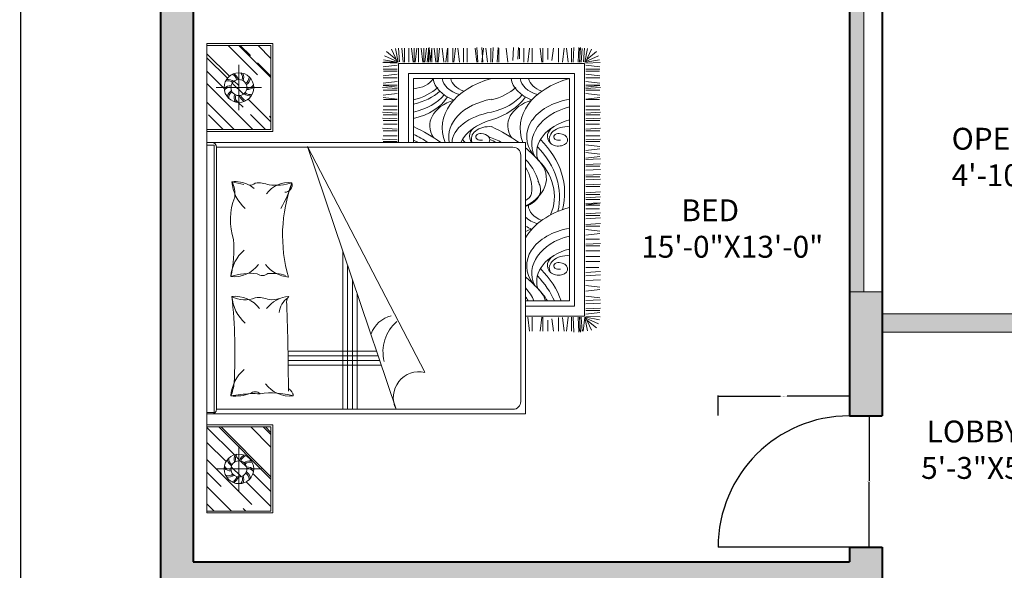
# Model space of a CAD drawing. Units: inches. Extents: x 2985 to 3527, y 3685 to 4528.
# Tile 3 of 5: x 2985 to 3255, y 4195 to 4346. Entities that reach past the tile are written whole.
import ezdxf

# ---------------------------------------------------------------- set-up
doc = ezdxf.new("R2010")
doc.units = ezdxf.units.IN
for name, color, linetype, lineweight in [('A-ANNO-DIMS', 2, 'Continuous', 18), ('A-AREA-IDEN', 7, 'Continuous', 25), ('A-FURN', 8, 'Continuous', 18), ('A-GLAZ', 4, 'Continuous', 18), ('A-WALL', 7, 'Continuous', 40), ('A-WALL-PATT', 8, 'Continuous', 13), ('door', 4, 'Continuous', 25)]:
    doc.layers.add(name, color=color, linetype=linetype, lineweight=lineweight)
doc.layers.add('A-GLAZ-PATT', color=241, linetype='Continuous', lineweight=13, true_color=0xf7abae)
doc.styles.get("Standard").update_dxf_attribs({"font": 'arial.ttf'})
doc.dimstyles.get("Standard").update_dxf_attribs({"dimtxt": 0.18, "dimasz": 0.18, "dimexe": 0.18, "dimexo": 0.0625, "dimgap": 0.09, "dimtad": 0, "dimtih": 1, "dimtoh": 1, "dimdec": 4, "dimzin": 0, "dimdsep": 46, "dimtxsty": 'Standard', "dimcen": 0.09, "dimadec": 0, "dimazin": 0, "dimtfac": 1, "dimtdec": 4, "dimtofl": 0, "dimtmove": 0, "dimatfit": 3, "dimfxl": 1, "dimtolj": 1, "dimtzin": 0, "dimarcsym": 0})

# ---------------------------------------------------------------- blocks, each defined once
blk = doc.blocks.new('A$C64B41DC1')
for p, q in [((0, 2.5079), (2.9903, 2.5079)), ((0, 2.0879), (0, 2.5079)), ((0.012, 2.4618), (0.0581, 2.5079)), ((0.012, 2.3515), (0.1684, 2.5079)), ((0.012, 2.0999), (0.012, 2.5079)), ((0.0543, 2.2213), (0.3409, 2.5079)), ((0.1689, 2.4179), (0.2589, 2.5079)), ((0.2804, 2.1597), (0.2804, 2.4481)), ((0.3265, 2.386), (0.4484, 2.5079)), ((0.3699, 2.3332), (0.5445, 2.5079)), ((0.548, 2.5079), (0.548, 2.0999)), ((0.56, 2.5079), (0.56, 2.0879)), ((0.6301, 2.5079), (0.6301, 0.4779)), ((0.6401, 2.461), (0.6401, 2.5079)), ((0.6401, 2.5079), (2.344, 2.5079)), ((2.344, 2.461), (0.6401, 2.461)), ((2.344, 2.5079), (2.3601, 2.5079)), ((2.344, 2.5079), (2.344, 2.461)), ((2.3601, 2.5079), (2.3601, 2.4761)), ((2.3601, 0.4779), (2.3601, 2.5079)), ((2.4303, 2.5079), (2.4303, 2.0879)), ((2.4423, 2.5079), (2.4423, 2.0999)), ((2.4423, 2.3333), (2.6169, 2.5079)), ((2.4423, 2.2145), (2.7357, 2.5079)), ((2.4423, 2.404), (2.5354, 2.4971)), ((2.705, 2.398), (2.8149, 2.5079)), ((2.7099, 2.1597), (2.7099, 2.4481)), ((2.7691, 2.3772), (2.8998, 2.5079)), ((2.7819, 2.3646), (2.9252, 2.5079)), ((2.9783, 2.0999), (2.9783, 2.5079)), ((2.9903, 2.0879), (2.9903, 2.5079)), ((0.2157, 2.0999), (0.548, 2.4322)), ((0.2299, 2.0999), (0.548, 2.418)), ((0.6601, 2.4461), (1.4951, 2.4461)), ((0.6601, 2.4461), (0.6601, 0.5579)), ((1.4951, 2.4461), (0.6697, 2.4461)), ((2.3301, 2.4461), (1.4951, 2.4461)), ((2.3301, 0.5579), (2.3301, 2.4461)), ((0.2311, 2.2906), (0.2937, 2.3532)), ((0.3405, 2.3039), (0.3605, 2.3238)), ((2.6158, 2.3088), (2.6313, 2.3243)), ((2.6674, 2.2756), (2.7382, 2.3464)), ((2.7249, 2.3076), (2.7512, 2.3339)), ((2.7914, 2.1846), (2.9783, 2.3715)), ((0.012, 2.261), (0.0275, 2.2765)), ((0.1362, 2.3039), (0.4246, 2.3039)), ((0.2905, 2.2539), (0.3304, 2.2938)), ((2.8541, 2.3039), (2.5657, 2.3039)), ((2.5849, 2.2779), (2.6158, 2.3088)), ((2.7746, 2.0999), (2.9783, 2.3036)), ((2.9144, 2.2312), (2.9783, 2.2951)), ((0.0404, 2.0999), (0.1982, 2.2578)), ((0.1365, 2.0999), (0.251, 2.2144)), ((0.4194, 2.0999), (0.548, 2.2285)), ((2.4423, 2.1353), (2.5382, 2.2312)), ((2.4918, 2.0999), (2.6366, 2.2447)), ((0.4986, 2.0999), (0.548, 2.1493)), ((0.5127, 2.0999), (0.548, 2.1352)), ((2.7831, 2.0999), (2.8678, 2.1846)), ((2.8962, 2.0999), (2.9783, 2.182)), ((0.56, 2.0879), (0, 2.0879)), ((0.548, 2.0999), (0.012, 2.0999)), ((2.4303, 2.0879), (2.9903, 2.0879)), ((2.4423, 2.0999), (2.9783, 2.0999)), ((2.5172, 2.0999), (2.5269, 2.1096)), ((0.9415, 1.9902), (0.9415, 1.3975)), ((0.9715, 1.9906), (0.9715, 1.4076)), ((1.0015, 1.991), (1.0015, 1.4177)), ((1.0315, 1.9916), (1.0315, 1.4279)), ((2.3349, 1.8678), (0.6613, 1.3029)), ((0.8956, 1.1191), (2.3349, 1.8678)), ((1.6636, 1.6412), (0.6601, 1.6412)), ((1.5748, 1.6112), (0.6601, 1.6112)), ((2.3665, 1.295), (2.3665, 1.3839)), ((2.377, 1.295), (2.3822, 1.3891)), ((2.4032, 1.295), (2.4032, 1.3839)), ((2.4346, 1.295), (2.4346, 1.3839)), ((2.4451, 1.295), (2.4503, 1.3891)), ((2.4774, 1.2957), (2.4774, 1.3837)), ((2.5, 1.295), (2.5, 1.3839)), ((2.5105, 1.295), (2.5157, 1.3891)), ((2.5367, 1.295), (2.5367, 1.3839)), ((2.5471, 1.295), (2.5524, 1.3891)), ((2.5681, 1.295), (2.5681, 1.3839)), ((2.5918, 1.295), (2.5918, 1.3839)), ((2.6346, 1.2957), (2.6346, 1.3837)), ((2.6362, 1.2957), (2.6467, 1.3839)), ((2.6729, 1.295), (2.6624, 1.3839)), ((2.6938, 1.295), (2.6938, 1.3839)), ((2.7043, 1.295), (2.7095, 1.3891)), ((2.7127, 1.2957), (2.7232, 1.3839)), ((2.7253, 1.295), (2.7253, 1.3839)), ((2.7494, 1.295), (2.7389, 1.3839)), ((2.7718, 1.295), (2.7718, 1.3839)), ((2.7959, 1.295), (2.7854, 1.3839)), ((2.8146, 1.2957), (2.8146, 1.3837)), ((2.8146, 1.2957), (2.8146, 1.3837)), ((2.8282, 1.295), (2.8282, 1.3839)), ((2.8282, 1.295), (2.8282, 1.3839)), ((2.8523, 1.295), (2.8418, 1.3839)), ((2.8523, 1.295), (2.8418, 1.3839)), ((2.8653, 1.2966), (2.8688, 1.3861)), ((2.8711, 1.2957), (2.8711, 1.3837)), ((2.8711, 1.2957), (2.8875, 1.3822)), ((2.8713, 1.2927), (2.954, 1.3315)), ((2.8765, 1.2958), (2.9132, 1.3758)), ((2.8893, 1.3011), (2.9394, 1.3636)), ((2.3601, 1.2873), (2.8639, 1.2873)), ((2.8639, 1.2873), (2.8639, 0.1018)), ((2.8716, 1.2565), (2.9605, 1.2669)), ((2.8717, 1.2884), (2.9588, 1.3058)), ((2.8744, 1.2817), (2.9603, 1.2869)), ((2.3601, 1.2233), (2.7999, 1.2233)), ((2.7999, 1.2233), (2.7999, 0.1658)), ((2.8716, 1.2212), (2.9605, 1.2212)), ((2.8716, 1.1947), (2.9605, 1.2052)), ((2.8723, 1.2489), (2.9603, 1.2489)), ((2.3601, 1.1913), (2.7679, 1.1912)), ((2.7679, 1.1912), (2.7679, 0.1978)), ((2.8716, 1.181), (2.9605, 1.1705)), ((2.8716, 1.1595), (2.9605, 1.1595)), ((2.8716, 1.133), (2.9605, 1.1435)), ((2.8723, 1.1872), (2.9603, 1.1872)), ((2.8716, 1.1193), (2.9605, 1.1088)), ((2.8716, 1.1035), (2.9605, 1.093)), ((2.8716, 1.0965), (2.9605, 1.0965)), ((2.8716, 1.086), (2.9657, 1.0913)), ((2.8716, 1.0756), (2.9605, 1.0756)), ((2.8723, 1.1255), (2.9603, 1.1255)), ((2.8723, 1.0858), (2.9605, 1.0753)), ((2.8716, 1.0491), (2.9605, 1.0596)), ((2.8716, 1.0354), (2.9605, 1.0249)), ((2.8723, 1.0416), (2.9603, 1.0416)), ((2.8723, 0.9987), (2.9605, 1.0092)), ((2.8723, 0.985), (2.9605, 0.9745)), ((2.8723, 0.9735), (2.9603, 0.9735)), ((2.8716, 0.9346), (2.9605, 0.9241)), ((2.8723, 0.9408), (2.9603, 0.9408)), ((2.8723, 0.8979), (2.9605, 0.9084)), ((2.8723, 0.8726), (2.9603, 0.8726)), ((2.8723, 0.8505), (2.9603, 0.8505)), ((2.8716, 0.7885), (2.9605, 0.799)), ((2.8716, 0.7818), (2.9657, 0.787)), ((2.8716, 0.7503), (2.9657, 0.7556)), ((2.8723, 0.7571), (2.9605, 0.7466)), ((2.8716, 0.7204), (2.9605, 0.7309)), ((2.8716, 0.6995), (2.9605, 0.6995)), ((2.8716, 0.689), (2.9657, 0.6838)), ((2.8716, 0.6576), (2.9657, 0.6523)), ((2.8716, 0.6471), (2.9605, 0.6471)), ((2.8716, 0.5903), (2.9605, 0.6007)), ((0.7101, 0.5079), (2.2801, 0.5079)), ((2.882, 0.5582), (2.9657, 0.5536)), ((2.8909, 0.5263), (2.9657, 0.5222)), ((2.8928, 0.5169), (2.9605, 0.5169)), ((0.6301, 0.4779), (2.3601, 0.4779)), ((1.2465, 0.4625), (1.1576, 0.452)), ((1.2542, 0.1018), (1.2542, 0.4779)), ((1.3182, 0.1658), (1.3182, 0.4779)), ((1.3502, 0.1978), (1.3502, 0.4779)), ((2.8716, 0.4877), (2.9603, 0.4877)), ((2.8716, 0.4625), (2.9605, 0.452)), ((1.2465, 0.3746), (1.1576, 0.3851)), ((1.2465, 0.4365), (1.1577, 0.4365)), ((2.8716, 0.4365), (2.9603, 0.4365)), ((2.8716, 0.3746), (2.9605, 0.3851)), ((1.2465, 0.3684), (1.1577, 0.3684)), ((1.2285, 0.3357), (1.1577, 0.3357)), ((2.8716, 0.3684), (2.9603, 0.3684)), ((2.8896, 0.3357), (2.9603, 0.3357)), ((1.2355, 0.3092), (1.1576, 0.3)), ((1.2457, 0.2676), (1.1577, 0.2676)), ((2.8723, 0.2676), (2.9603, 0.2676)), ((2.8826, 0.3092), (2.9605, 0.3)), ((1.2457, 0.2423), (1.1576, 0.2319)), ((1.2465, 0.2057), (1.1576, 0.2161)), ((2.7679, 0.1978), (1.3502, 0.1978)), ((2.8716, 0.2057), (2.9605, 0.2161)), ((2.8723, 0.2423), (2.9605, 0.2319)), ((1.2465, 0.1742), (1.1524, 0.169)), ((1.2465, 0.1428), (1.1524, 0.1376)), ((1.2465, 0.1334), (1.1524, 0.1281)), ((1.2465, 0.1847), (1.1576, 0.1847)), ((1.2465, 0.1323), (1.1576, 0.1323)), ((1.2465, 0.1323), (1.1576, 0.1323)), ((2.7999, 0.1658), (1.3182, 0.1658)), ((2.8716, 0.1847), (2.9605, 0.1847)), ((2.8716, 0.1742), (2.9657, 0.169)), ((2.8716, 0.1428), (2.9657, 0.1376)), ((2.8716, 0.1334), (2.9657, 0.1281)), ((2.8716, 0.1323), (2.9605, 0.1323)), ((1.2465, 0.1), (1.1576, 0.1105)), ((1.2465, 0.1229), (1.1588, 0.1168)), ((1.2464, 0.1007), (1.1592, 0.0833)), ((1.2468, 0.0964), (1.1641, 0.0576)), ((1.2288, 0.088), (1.1787, 0.0255)), ((1.2415, 0.0933), (1.2049, 0.0133)), ((1.247, 0.0934), (1.2306, 0.0069)), ((1.2527, 0.0925), (1.2493, 0.003)), ((2.8639, 0.1018), (1.2542, 0.1018)), ((1.2658, 0.0941), (1.2762, 0.0052)), ((1.2899, 0.0941), (1.2899, 0.0052)), ((1.2999, 0.0941), (1.3051, 0)), ((1.3313, 0.0941), (1.3365, 0)), ((1.3523, 0.0941), (1.3575, 0)), ((1.3804, 0.0941), (1.3699, 0.0052)), ((1.4119, 0.0934), (1.4223, 0.0052)), ((1.4485, 0.0941), (1.438, 0.0052)), ((1.48, 0.0941), (1.4852, 0)), ((1.5114, 0.0941), (1.5166, 0)), ((1.5323, 0.0941), (1.5376, 0)), ((1.5638, 0.0941), (1.5638, 0.0105)), ((1.6021, 0.0941), (1.6021, 0.0052)), ((1.6336, 0.0941), (1.6336, 0.0052)), ((1.6702, 0.0941), (1.6702, 0.0052)), ((1.7017, 0.0941), (1.7017, 0.0052)), ((1.7122, 0.0941), (1.7174, 0)), ((1.7445, 0.0934), (1.7445, 0.0054)), ((1.7698, 0.0934), (1.7803, 0.0052)), ((1.8065, 0.0941), (1.796, 0.0052)), ((1.8274, 0.0941), (1.8274, 0.0052)), ((1.8379, 0.0941), (1.8431, 0)), ((1.8746, 0.0941), (1.8798, 0)), ((1.8955, 0.0941), (1.8955, 0.0052)), ((1.906, 0.0941), (1.9113, 0)), ((1.9384, 0.0934), (1.9384, 0.0054)), ((1.9609, 0.0941), (1.9609, 0.0052)), ((1.9636, 0.0934), (1.9741, 0.0052)), ((1.9714, 0.0941), (1.9766, 0)), ((1.9976, 0.0941), (1.9976, 0.0052)), ((2.0081, 0.0941), (2.0133, 0)), ((2.029, 0.0941), (2.029, 0.0052)), ((2.0395, 0.0941), (2.0447, 0)), ((2.0797, 0.0941), (2.0797, 0.0052)), ((2.0902, 0.0941), (2.0954, 0)), ((2.1216, 0.0941), (2.1269, 0)), ((2.1412, 0.0941), (2.1412, 0.0052)), ((2.1517, 0.0941), (2.1569, 0)), ((2.1831, 0.0941), (2.1884, 0)), ((2.2093, 0.0941), (2.2093, 0.0052)), ((2.2198, 0.0941), (2.225, 0)), ((2.2512, 0.0941), (2.2565, 0)), ((2.2603, 0.0934), (2.2707, 0.0052)), ((2.2969, 0.0941), (2.2864, 0.0052)), ((2.3089, 0.0934), (2.3193, 0.0052)), ((2.3455, 0.0941), (2.3351, 0.0052)), ((2.3665, 0.0941), (2.3665, 0.0052)), ((2.377, 0.0941), (2.3822, 0)), ((2.4032, 0.0941), (2.4032, 0.0052)), ((2.4346, 0.0941), (2.4346, 0.0052)), ((2.4451, 0.0941), (2.4503, 0)), ((2.4774, 0.0934), (2.4774, 0.0054)), ((2.5, 0.0941), (2.5, 0.0052)), ((2.5105, 0.0941), (2.5157, 0)), ((2.5367, 0.0941), (2.5367, 0.0052)), ((2.5471, 0.0941), (2.5524, 0)), ((2.5681, 0.0941), (2.5681, 0.0052)), ((2.5918, 0.0941), (2.5918, 0.0052)), ((2.6346, 0.0934), (2.6346, 0.0054)), ((2.6362, 0.0934), (2.6467, 0.0052)), ((2.6729, 0.0941), (2.6624, 0.0052)), ((2.6938, 0.0941), (2.6938, 0.0052)), ((2.7043, 0.0941), (2.7095, 0)), ((2.7127, 0.0934), (2.7232, 0.0052)), ((2.7253, 0.0941), (2.7253, 0.0052)), ((2.7494, 0.0941), (2.7389, 0.0052)), ((2.7718, 0.0941), (2.7718, 0.0052)), ((2.7959, 0.0941), (2.7854, 0.0052)), ((2.8146, 0.0934), (2.8146, 0.0054)), ((2.8282, 0.0941), (2.8282, 0.0052)), ((2.8523, 0.0941), (2.8418, 0.0052)), ((2.8653, 0.0925), (2.8688, 0.003)), ((2.8711, 0.0934), (2.8875, 0.0069)), ((2.8713, 0.0964), (2.954, 0.0576)), ((2.8716, 0.1229), (2.9593, 0.1168)), ((2.8717, 0.1007), (2.9588, 0.0833)), ((2.8744, 0.1074), (2.9603, 0.1022)), ((2.8765, 0.0933), (2.9132, 0.0133)), ((2.8893, 0.088), (2.9394, 0.0255))]:
    blk.add_line(p, q)
at = {"ltscale": 10}
for p, q in [((1.4859, 1.5812), (0.6601, 1.5812)), ((1.397, 1.5512), (0.6601, 1.5512))]:
    blk.add_line(p, q, dxfattribs=at)
for centre, radius in [((0.2804, 2.3039), 0.0942), ((2.7099, 2.3039), 0.0942), ((0.2804, 2.3039), 0.051), ((2.7099, 2.3039), 0.051)]:
    blk.add_circle(centre, radius)
for centre, radius, start, end in [((0.6601, 2.4761), 0.03, 180, 270), ((2.3301, 2.4761), 0.03, 270, 0), ((0.2828, 2.3731), 0.0462, 160.30017, 220.53802), ((0.3286, 2.3561), 0.0605, 136.17003, 182.48975), ((0.3231, 2.3585), 0.0462, 124.30017, 184.53802), ((2.6672, 2.3585), 0.0462, 355.46198, 55.69983), ((2.6617, 2.3561), 0.0605, 357.51025, 43.82997), ((2.7075, 2.3731), 0.0462, 319.46198, 19.69983), ((0.2457, 2.3659), 0.0605, 208.17003, 254.48975), ((0.2417, 2.3614), 0.0462, 196.30017, 256.53802), ((0.2887, 2.3745), 0.0605, 172.17003, 218.48975), ((0.3501, 2.3178), 0.0605, 100.17003, 146.48975), ((0.347, 2.323), 0.0462, 88.30017, 148.53802), ((0.3449, 2.2742), 0.0605, 64.17003, 110.48975), ((0.3455, 2.2802), 0.0462, 52.30017, 112.53802), ((1.0526, 2.3302), 0.3085, 175.30484, 198.69419), ((-0.8702, 2.0941), 1.6364, 4.80985, 9.18918), ((0.8579, 2.6278), 0.2948, 247.51785, 264.26696), ((0.728, 2.111), 0.245, 40.4189, 85.9871), ((1.0164, 5.7096), 3.3803, 266.81337, 276.16021), ((1.3963, 2.1044), 0.245, 94.0129, 139.5811), ((1.1858, 2.3288), 0.1943, 306.5711, 5.88998), ((1.5348, 2.2652), 0.1767, 151.77364, 201.69827), ((1.6986, 2.3355), 0.1943, 174.11002, 233.4289), ((1.1481, 2.2311), 0.3783, 353.49469, 19.18669), ((1.6871, 3.192), 0.8561, 257.74383, 273.62843), ((1.4882, 2.111), 0.245, 40.4189, 85.9871), ((1.8674, 1.9709), 0.3878, 68.20259, 108.9817), ((2.1269, 2.1044), 0.245, 94.0129, 139.5811), ((2.0342, 2.4856), 0.1563, 261.59582, 298.90918), ((1.9165, 2.3288), 0.1943, 333.73715, 5.88998), ((2.6058, 2.2028), 0.517, 163.60457, 172.3273), ((2.6448, 2.2802), 0.0462, 67.46198, 127.69983), ((2.6454, 2.2742), 0.0605, 69.51025, 115.82997), ((2.6433, 2.323), 0.0462, 31.46198, 91.69983), ((2.6402, 2.3178), 0.0605, 33.51025, 79.82997), ((2.7016, 2.3745), 0.0605, 321.51025, 7.82997), ((2.7486, 2.3614), 0.0462, 283.46198, 343.69983), ((2.7446, 2.3659), 0.0605, 285.51025, 331.82997), ((0.2153, 2.3276), 0.0462, 232.30017, 292.53802), ((0.2158, 2.3336), 0.0605, 244.17003, 290.48975), ((0.2138, 2.2848), 0.0462, 268.30017, 328.53802), ((0.2779, 2.2347), 0.0462, 340.30017, 40.53802), ((0.272, 2.2333), 0.0605, 352.17003, 38.48975), ((0.3191, 2.2464), 0.0462, 16.30017, 76.53802), ((0.3151, 2.2419), 0.0605, 28.17003, 74.48975), ((2.6752, 2.2419), 0.0605, 105.51025, 151.82997), ((2.6712, 2.2464), 0.0462, 103.46198, 163.69983), ((2.7182, 2.2333), 0.0605, 141.51025, 187.82997), ((2.7123, 2.2347), 0.0462, 139.46198, 199.69983), ((2.7765, 2.2848), 0.0462, 211.46198, 271.69983), ((2.7744, 2.3336), 0.0605, 249.51025, 295.82997), ((2.775, 2.3276), 0.0462, 247.46198, 307.69983), ((0.2107, 2.29), 0.0605, 280.17003, 326.48975), ((0.2377, 2.2493), 0.0462, 304.30017, 4.53802), ((0.2322, 2.2517), 0.0605, 316.17003, 2.48975), ((0.7274, 2.2013), 0.0446, 314.4736, 42.17134), ((-1.6008, 2.277), 2.3618, 357.39054, 358.88764), ((1.204, 2.1778), 0.1681, 337.01697, 7.53676), ((1.9165, 2.3288), 0.1943, 320.94042, 333.73715), ((2.1347, 2.2313), 0.0459, 165.35061, 223.26844), ((1.9346, 2.1778), 0.1681, 337.01697, 7.53676), ((2.7581, 2.2517), 0.0605, 177.51025, 223.82997), ((2.7526, 2.2493), 0.0462, 175.46198, 235.69983), ((2.7796, 2.29), 0.0605, 213.51025, 259.82997), ((0.9385, 1.978), 0.1943, 126.5711, 185.88998), ((0.2688, 2.0945), 0.4956, 344.0243, 8.70709), ((1.7059, 1.9714), 0.204, 127.11975, 175.09005), ((1.5671, 2.1546), 0.0547, 142.08329, 220.902), ((1.1858, 1.9714), 0.1943, 4.31813, 53.4289), ((1.5415, 2.0969), 0.1834, 175.22328, 196.23004), ((1.1965, 2.0983), 0.3299, 343.79543, 3.55541), ((1.9394, 1.991), 0.1651, 351.26213, 55.75721), ((2.4617, 2.0719), 0.3745, 173.82958, 196.4356), ((1.2687, 1.9248), 0.1223, 33.62799, 86.47438), ((1.7676, 1.0629), 0.9631, 69.65065, 105.96307), ((2.2748, 2.5795), 0.6373, 238.34989, 254.31375), ((2.0911, 2.0123), 0.0478, 179.77267, 283.80184), ((0.7417, 2.0149), 0.057, 273.47085, 328.54118), ((0.728, 2.2025), 0.245, 274.0129, 278.34166), ((0.7246, 18.8439), 16.8552, 270.17399, 272.05214), ((1.3401, 1.9404), 0.0603, 49.09906, 101.37023), ((1.0747, 1.2871), 0.1871, 14.1863, 69.12121), ((1.0274, 1.1334), 0.2527, 40.62904, 104.37123), ((0.7347, 1.1553), 0.1649, 347.31088, 116.44537), ((0.7101, 0.5579), 0.05, 180, 270), ((2.2801, 0.5579), 0.05, 270, 0)]:
    blk.add_arc(centre, radius, start, end)
for centre, major_axis, ratio, start_param, end_param in [((1.9938, 1.6262), (0, -0.7531), 0.68, 0.797284, 0.954936), ((2.0643, 1.466), (0, -0.5322), 0.68, 7.239912, 7.311536), ((1.9052, 1.7397), (0, -0.9842), 0.68, 0.74745, 0.979724), ((2.7455, 1.3081), (0, 0.3614), 0.68, 1.900046, 2.742661), ((2.7868, 1.3081), (0, 0.3614), 0.68, 1.900046, 2.614747), ((2.8372, 1.3081), (0, 0.3614), 0.68, 1.900046, 2.479658), ((2.8607, 1.3211), (0, 0.3614), 0.68, 1.938265, 2.479658), ((2.8057, 1.2079), (0, -0.1524), 0.68, 4.821745, 5.895886), ((2.4665, 0.8216), (0, -0.2664), 0.68, 2.006169, 3.565187), ((2.7862, 0.8069), (0, -0.2615), 0.68, 3.244645, 4.205018), ((2.4513, 0.5069), (0, 0.502), 0.68, 5.095327, 6.553458), ((2.7784, 0.8289), (0, -0.1802), 0.68, 3.227058, 4.318474), ((2.396, 0.6032), (0, 0.3641), 0.68, -1.3172, 0.145284), ((2.3507, 0.5642), (0.0073, 0.3819), 0.56205, -1.21172, -0.009991), ((2.7821, 0.7971), (0, -0.1589), 0.68, 3.272942, 4.229533), ((2.2964, 0.5771), (0, -0.3263), 0.68, 1.938944, 2.850232), ((2.0403, 1.6015), (0, -0.8763), 0.68, 6.849801, 6.887077), ((2.4005, 0.7132), (0, -0.1214), 0.68, 2.284368, 3.652258), ((2.3834, 0.7081), (0, 0.1147), 0.68, 4.593909, 6.585576), ((2.3774, 0.7653), (0, -0.0593), 0.68, 5.841311, 7.755362), ((2.3961, 0.7628), (0, -0.0317), 0.68, 1.462497, 5.046281), ((1.9938, 1.1295), (-0.0678, 0.7439), 0.610498, 3.917146, 4.063997), ((2.0643, 0.9693), (0, -0.5322), 0.68, 7.239912, 7.336618), ((1.9052, 1.243), (0, -0.9842), 0.68, 0.74745, 0.979724), ((2.7455, 0.8114), (-0.0599, 0.3735), 0.695517, 1.775813, 2.548612), ((2.7868, 0.8114), (0, 0.3614), 0.68, 1.900046, 2.614747), ((2.8607, 0.8243), (0, 0.3614), 0.68, 1.938265, 2.479658), ((2.4665, 0.3249), (0, -0.2664), 0.68, 2.006169, 3.565187), ((2.7862, 0.3102), (0, -0.2615), 0.68, 3.244645, 4.205018), ((2.4513, 0.0102), (0, 0.502), 0.68, 5.095327, 6.553458), ((2.7784, 0.3322), (0, -0.1802), 0.68, 3.227058, 4.318474), ((1.242, 0.9693), (0, -0.5322), 0.68, 6.586764, 6.677612), ((1.1714, 1.1295), (-0.1157, 0.7241), 0.59432, 3.291697, 3.50733), ((1.0828, 1.243), (0, -0.9842), 0.68, 0.565948, 0.680366), ((1.5283, 0.0674), (0, -0.3703), 0.68, 1.930561, 3.464283), ((1.5736, 0.1065), (0, 0.3641), 0.68, -1.3172, 0.476403), ((1.6289, 0.0102), (0, 0.502), 0.68, 6.655152, 6.661293), ((1.6289, 0.0102), (0, 0.502), 0.68, 5.095327, 5.911219), ((1.6442, 0.3249), (0, -0.2664), 0.68, 2.006169, 2.182797), ((1.9638, 0.3102), (0, -0.2615), 0.68, 4.015924, 4.205018), ((1.956, 0.3322), (0, -0.1802), 0.68, 3.770744, 4.318474), ((1.9597, 0.3004), (0, -0.1589), 0.68, 3.14258, 4.229533), ((2.0606, 0.5616), (0, -0.1803), 0.68, 5.194792, 5.929328), ((2.0606, 0.5616), (0, -0.1803), 0.68, 5.194792, 6.723255), ((2.1315, 0.6603), (0, -0.3155), 0.68, 5.328638, 6.949396), ((2.0549, 0.5656), (0, -0.1303), 0.68, 5.450951, 6.054641), ((2.0643, 0.9693), (0, -0.5322), 0.68, 6.20013, 6.677612), ((1.9938, 1.1295), (-0.0678, 0.7439), 0.610498, 3.199135, 3.592282), ((1.9052, 1.243), (0, -0.9842), 0.68, 0.565948, 0.680366), ((2.3507, 0.0674), (0, -0.3703), 0.68, 1.930561, 3.464283), ((2.396, 0.1065), (0, 0.3641), 0.68, -1.3172, 0.476403), ((2.4513, 0.0102), (0, 0.502), 0.68, 6.655152, 6.661293), ((2.7821, 0.3004), (0, -0.1589), 0.68, 3.272942, 4.229533), ((1.1933, 0.9181), (0, -0.624), 0.68, 0.378672, 0.625379), ((1.3091, 0.6603), (0, -0.3155), 0.68, 6.475719, 6.949396), ((1.1911, 1.1066), (0, 0.8458), 0.68, 3.421828, 3.728616), ((1.2179, 1.1047), (0, -0.8763), 0.68, 6.507006, 6.887077), ((1.474, 0.0804), (0, -0.3263), 0.68, 1.938944, 3.339184), ((2.0157, 0.9181), (0, -0.624), 0.68, -0.280078, 0.625379), ((2.0135, 1.1066), (0, 0.8458), 0.68, 2.978727, 3.728616), ((2.0403, 1.1047), (0, -0.8763), 0.68, 6.099302, 6.887077), ((2.2964, 0.0804), (0, -0.3263), 0.68, 1.938944, 3.339184), ((1.555, 0.2685), (0, -0.0593), 0.68, 3.732151, 7.755362), ((1.5781, 0.2165), (0, -0.1214), 0.68, 2.284368, 3.726131), ((1.561, 0.2114), (0, 0.1147), 0.68, 4.593909, 6.647252), ((2.3774, 0.2685), (0, -0.0593), 0.68, 3.732151, 7.755362), ((2.4005, 0.2165), (0, -0.1214), 0.68, 2.284368, 3.726131), ((2.3834, 0.2114), (0, 0.1147), 0.68, 4.593909, 6.647252), ((1.5737, 0.2661), (0, -0.0317), 0.68, 1.462497, 5.046281), ((2.3961, 0.2661), (0, -0.0317), 0.68, 1.462497, 5.046281)]:
    blk.add_ellipse(centre, major_axis=major_axis, ratio=ratio, start_param=start_param, end_param=end_param)
blk = doc.blocks.new('DOOR-SWING-36IN')
blk.add_line((0, 0), (0, 36))
blk.add_arc((0, 0), 36, 0, 90)
blk = doc.blocks.new('*D18')
at = {"layer": 'A-ANNO-DIMS', "color": 0, "lineweight": -2, "transparency": 16777216}
for p, q in [((3176.83, 4237.43), (3176.83, 4242.95)), ((3177.01, 4242.77), (3193.9, 4242.77)), ((3212.65, 4242.77), (3195.77, 4242.77)), ((3212.83, 4237.43), (3212.83, 4242.95))]:
    blk.add_line(p, q, dxfattribs=at)
at = {"layer": 'A-ANNO-DIMS', "color": 0, "transparency": 16777216}
for points in [[(3177.01, 4242.8), (3177.01, 4242.74), (3176.83, 4242.77)], [(3212.65, 4242.8), (3212.65, 4242.74), (3212.83, 4242.77)]]:
    blk.add_solid(points, dxfattribs=at)
at = {"layer": 'Defpoints', "color": 0, "transparency": 16777216}
for p in [(3176.83, 4242.77), (3176.83, 4237.37), (3212.83, 4237.37)]:
    blk.add_point(p, dxfattribs=at)
at = {"layer": 'A-ANNO-DIMS', "color": 0, "transparency": 16777216, "insert": (3194.83, 4242.77), "char_height": 0.18, "attachment_point": 5}
blk.add_mtext('\\A1;DOOR 36 TYP.', dxfattribs=at)
blk = doc.blocks.new('*D19')
at = {"layer": 'A-ANNO-DIMS', "color": 0, "lineweight": -2, "transparency": 16777216}
for p, q in [((3212.9, 4237.37), (3218.41, 4237.37)), ((3218.23, 4237.19), (3218.23, 4219.55)), ((3218.23, 4201.55), (3218.23, 4219.19)), ((3212.9, 4201.37), (3218.41, 4201.37))]:
    blk.add_line(p, q, dxfattribs=at)
at = {"layer": 'A-ANNO-DIMS', "color": 0, "transparency": 16777216}
for points in [[(3218.2, 4237.19), (3218.26, 4237.19), (3218.23, 4237.37)], [(3218.2, 4201.55), (3218.26, 4201.55), (3218.23, 4201.37)]]:
    blk.add_solid(points, dxfattribs=at)
at = {"layer": 'Defpoints', "color": 0, "transparency": 16777216}
for p in [(3212.83, 4237.37), (3218.23, 4237.37), (3212.83, 4201.37)]:
    blk.add_point(p, dxfattribs=at)
at = {"layer": 'A-ANNO-DIMS', "color": 0, "transparency": 16777216, "insert": (3218.23, 4219.37), "char_height": 0.18, "attachment_point": 5}
blk.add_mtext('\\A1;36 TYP.', dxfattribs=at)
blk = doc.blocks.new('*D41')
at = {"layer": 'A-ANNO-DIMS', "color": 0, "lineweight": -2, "transparency": 16777216}
for p, q in [((3023.77, 4439.37), (2985.25, 4439.37)), ((2985.43, 4439.19), (2985.43, 4081.55)), ((2985.43, 3723.55), (2985.43, 4081.19)), ((3023.77, 3723.37), (2985.25, 3723.37))]:
    blk.add_line(p, q, dxfattribs=at)
at = {"layer": 'A-ANNO-DIMS', "color": 0, "transparency": 16777216}
for points in [[(2985.4, 4439.19), (2985.46, 4439.19), (2985.43, 4439.37)], [(2985.4, 3723.55), (2985.46, 3723.55), (2985.43, 3723.37)]]:
    blk.add_solid(points, dxfattribs=at)
at = {"layer": 'Defpoints', "color": 0, "transparency": 16777216}
for p in [(2985.43, 4439.37), (3023.83, 4439.37), (3023.83, 3723.37)]:
    blk.add_point(p, dxfattribs=at)
at = {"layer": 'A-ANNO-DIMS', "color": 0, "transparency": 16777216, "insert": (2985.43, 4081.37), "char_height": 0.18, "attachment_point": 5}
blk.add_mtext('\\A1;716', dxfattribs=at)

msp = doc.modelspace()

# ---------------------------------------------------------------- hatches: boundary and pattern name
at = {"layer": 'A-GLAZ-PATT'}
h = msp.add_hatch(color=256, dxfattribs=at)
h.dxf.hatch_style = 1
h.paths.add_polyline_path([(3216.833, 4349.372), (3212.833, 4349.372), (3212.833, 4271.372), (3216.833, 4271.372)])
h.paths.add_polyline_path([(3250.833, 4358.372), (3221.833, 4358.372), (3221.833, 4354.372), (3250.833, 4354.372)])
h.paths.add_polyline_path([(3290.333, 4358.372), (3259.833, 4358.372), (3259.833, 4354.372), (3290.333, 4354.372)])
h.paths.add_polyline_path([(3299.333, 4349.372), (3295.333, 4349.372), (3295.333, 4271.372), (3299.333, 4271.372)])
h.paths.add_polyline_path([(3290.333, 4265.372), (3221.833, 4265.372), (3221.833, 4260.372), (3290.333, 4260.372)])
at = {"layer": 'A-WALL-PATT'}
h = msp.add_hatch(color=256, dxfattribs=at)
h.dxf.hatch_style = 1
h.paths.add_polyline_path([(3023.833, 4065.372), (3023.833, 3771.372), (3111.083, 3771.372), (3111.083, 3780.372), (3032.833, 3780.372), (3032.833, 3936.372), (3221.333, 3936.372), (3221.333, 3945.372), (3215.333, 3945.372), (3215.333, 3981.372), (3206.333, 3981.372), (3206.333, 3945.372), (3032.833, 3945.372), (3032.833, 4065.372), (3079.333, 4065.372), (3079.333, 4074.372), (3032.833, 4074.372), (3032.833, 4188.372), (3119.333, 4188.372), (3119.333, 4107.372), (3215.333, 4107.372), (3215.333, 4148.372), (3206.333, 4148.372), (3206.333, 4116.372), (3124.333, 4116.372), (3124.333, 4188.372), (3206.333, 4188.372), (3206.333, 4184.372), (3215.333, 4184.372), (3215.333, 4188.372), (3221.833, 4188.372), (3221.833, 4201.372), (3212.833, 4201.372), (3212.833, 4197.372), (3032.833, 4197.372), (3032.833, 4353.372), (3068.479, 4353.372), (3068.479, 4358.372), (3032.833, 4358.372), (3032.833, 4430.372), (3137.833, 4430.372), (3137.833, 4404.372), (3137.833, 4392.372), (3142.833, 4392.372), (3142.833, 4430.372), (3190.833, 4430.372), (3190.833, 4439.372), (3023.833, 4439.372)])
h = msp.add_hatch(color=256, dxfattribs=at)
h.dxf.hatch_style = 1
h.paths.add_polyline_path([(3221.833, 4271.372), (3212.833, 4271.372), (3212.833, 4237.372), (3221.833, 4237.372)])
h.paths.add_polyline_path([(3299.333, 4271.372), (3290.333, 4271.372), (3290.333, 4249.372), (3299.333, 4249.372)])

# ---------------------------------------------------------------- linework, layer by layer
at = {"layer": 'A-GLAZ'}
for p, q in [((3216.833, 4349.372), (3216.833, 4271.372)), ((3212.833, 4271.372), (3221.833, 4271.372)), ((3221.833, 4265.372), (3290.333, 4265.372)), ((3221.833, 4260.372), (3290.333, 4260.372))]:
    msp.add_line(p, q, dxfattribs=at)
at = {"layer": 'A-WALL'}
for p, q in [((3023.833, 4439.372), (3023.833, 4065.372)), ((3221.833, 4358.372), (3221.833, 4237.372)), ((3032.833, 4353.372), (3032.833, 4197.372)), ((3212.833, 4353.372), (3212.833, 4237.372)), ((3212.833, 4237.372), (3221.833, 4237.372)), ((3212.833, 4201.372), (3221.833, 4201.372)), ((3212.833, 4201.372), (3212.833, 4197.372)), ((3221.833, 4201.372), (3221.833, 4188.372)), ((3032.833, 4197.372), (3212.833, 4197.372))]:
    msp.add_line(p, q, dxfattribs=at)

# ---------------------------------------------------------------- block references
at = {"layer": 'A-FURN', "xscale": 43.05186407285219, "yscale": 43.05186407285219, "zscale": 43.05186407285219, "rotation": 90}
msp.add_blockref('A$C64B41DC1', (3144.56, 4210.755), dxfattribs=at)
at = {"layer": 'door', "rotation": 90.00000000000179}
msp.add_blockref('DOOR-SWING-36IN', (3212.833, 4201.372), dxfattribs=at)

# ---------------------------------------------------------------- texts
at = {"layer": 'A-AREA-IDEN', "attachment_point": 1}
for s, width, insert, char_height in [('OPEN \\P4\'-10.5"X7\'', 31.7894, (3240.887, 4316.386), 6), ('      BED\\P15\'-0"X13\'-0"', 31.99995, (3155.732, 4296.759), 6), ('  {\\H2.4x;LOBBY\\P5\'-3"X5\'-0"}', 56.03015, (3232.521, 4236.086), 2.5)]:
    msp.add_mtext_dynamic_manual_height_columns(s, width=width, gutter_width=12.5, heights=[0], dxfattribs=dict(at, insert=insert, char_height=char_height))

# ---------------------------------------------------------------- dimensions: what is measured, and where the dimension line sits
at = {"layer": 'A-ANNO-DIMS'}
dim = msp.add_linear_dim(base=(2985.433, 4439.372), p1=(3023.833, 3723.372), p2=(3023.833, 4439.372), angle=90, dimstyle='Standard', override={"dimdec": 0, "dimlfac": 1, "dimrnd": 0, "dimzin": 0, "dimdsep": 46, "dimlunit": 2}, dxfattribs=at)
dim.commit()
dim.dimension.update_dxf_attribs({"geometry": '*D41', "text_midpoint": (2985.433, 4081.372)})
for base, p1, p2, angle, text, picture, middle in [((3176.833, 4242.772), (3212.833, 4237.372), (3176.833, 4237.372), 180, 'DOOR <> TYP.', '*D18', (3194.833, 4242.772)), ((3218.233, 4237.372), (3212.833, 4201.372), (3212.833, 4237.372), 90, '<> TYP.', '*D19', (3218.233, 4219.372))]:
    dim = msp.add_linear_dim(base=base, p1=p1, p2=p2, angle=angle, text=text, dimstyle='Standard', override={"dimdec": 0, "dimlfac": 1, "dimrnd": 0, "dimzin": 0, "dimdsep": 46, "dimlunit": 2}, dxfattribs=at)
    dim.commit()
    dim.dimension.update_dxf_attribs({"geometry": picture, "text_midpoint": middle})

doc.saveas('drawing.dxf')
